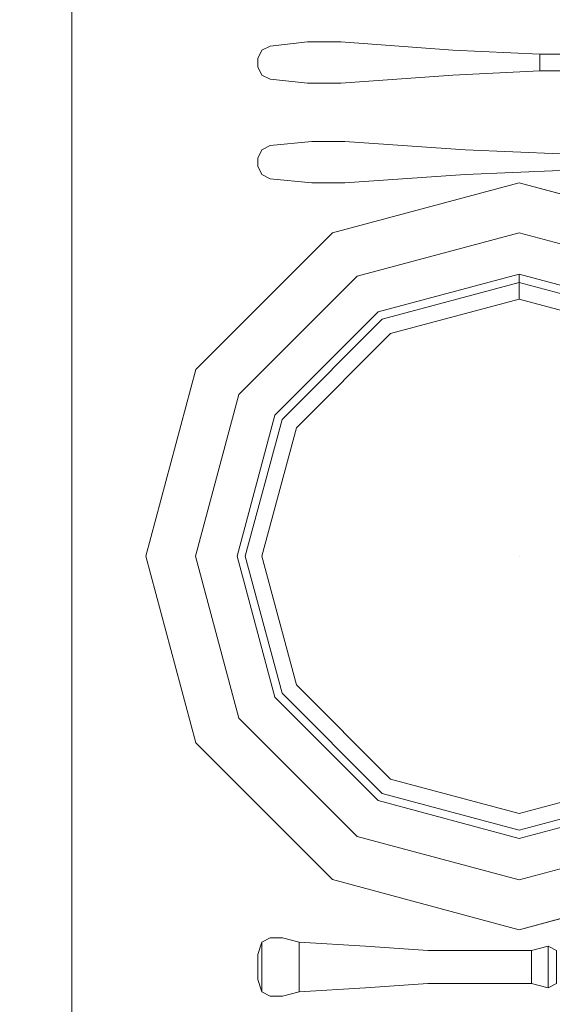
# Model space of a CAD drawing. Units: inches. Extents: x 375 to 1122, y 27 to 1069.
# Tile 18 of 155: x 705.14 to 713.05, y 270.59 to 285.2. Entities that reach past the tile are written whole.
import ezdxf

# ---------------------------------------------------------------- set-up
doc = ezdxf.new("R2010")
doc.units = ezdxf.units.IN
doc.layers.add('A-ANNO-DIMS', color=2, linetype='Continuous', lineweight=18)
doc.layers.add('Furniture', color=30, linetype='Continuous', lineweight=18)
doc.styles.get("Standard").update_dxf_attribs({"font": 'arial.ttf'})
doc.dimstyles.new('ISO-25', dxfattribs={"dimtxt": 12, "dimasz": 2.5, "dimexe": 1.5, "dimexo": 1.5, "dimtad": 1, "dimdec": 1, "dimlunit": 3, "dimtxsty": 'Standard', "dimblk": 'ARCHTICK', "dimcen": 2.5, "dimadec": 0, "dimazin": 0, "dimtfac": 1, "dimtdec": 1, "dimtmove": 0, "dimatfit": 3, "dimfxl": 1.5, "dimfxlon": 1, "dimarcsym": 0})

# ---------------------------------------------------------------- blocks, each defined once
blk = doc.blocks.new('A$C403C54AD')
blk.add_line((0.83575, 0.52421, -0.0006), (1.99923, 0.52421, -0.0006))
at = {"linetype": 'ByBlock'}
for points, invisible_edges in [([(1.72651, 0.7917, -0.01489), (1.72651, 0.69011, -0.01489), (1.72651, 0.69011, -0.01489), (1.67572, 0.77809, -0.01489)], 5), ([(1.7773, 0.77809, -0.01489), (1.72651, 0.69011, -0.01489), (1.72651, 0.69011, -0.01489), (1.72651, 0.7917, -0.01489)], 5), ([(1.67572, 0.77809, -0.01489), (1.72651, 0.69011, -0.01489), (1.72651, 0.69011, -0.01489), (1.63853, 0.74091, -0.01489)], 5), ([(1.81449, 0.74091, -0.01489), (1.72651, 0.69011, -0.01489), (1.72651, 0.69011, -0.01489), (1.7773, 0.77809, -0.01489)], 5), ([(1.60654, 0.75938, -0.00874), (1.62254, 0.75014, -0.00874), (1.60645, 0.69011, -0.00874), (1.58798, 0.69011, -0.00874)], 5), ([(1.63587, 0.74244, -0.02259), (1.60654, 0.75938, -0.01335), (1.58798, 0.69011, -0.01335), (1.62185, 0.69011, -0.02259)], 5), ([(1.83118, 0.69011, -0.02259), (1.86504, 0.69011, -0.01335), (1.84648, 0.75938, -0.01335), (1.81715, 0.74244, -0.02259)], 5), ([(1.86504, 0.69011, -0.00874), (1.84657, 0.69011, -0.00874), (1.83048, 0.75014, -0.00874), (1.84648, 0.75938, -0.00874)], 5), ([(1.62254, 0.75014, -0.00874), (1.63853, 0.74091, -0.01489), (1.62492, 0.69011, -0.01489), (1.60645, 0.69011, -0.00874)], 5), ([(1.84657, 0.69011, -0.00874), (1.8281, 0.69011, -0.01489), (1.81449, 0.74091, -0.01489), (1.83048, 0.75014, -0.00874)], 5), ([(1.82194, 0.69011, -0.03183), (1.83118, 0.69011, -0.02259), (1.81715, 0.74244, -0.02259), (1.80916, 0.73783, -0.03183)], 5), ([(1.63853, 0.74091, -0.01489), (1.72651, 0.69011, -0.01489), (1.72651, 0.69011, -0.01489), (1.62492, 0.69011, -0.01489)], 5), ([(1.8281, 0.69011, -0.01489), (1.72651, 0.69011, -0.01489), (1.72651, 0.69011, -0.01489), (1.81449, 0.74091, -0.01489)], 5), ([(1.58798, 0.69011, -0.00874), (1.60645, 0.69011, -0.00874), (1.62254, 0.63008, -0.00874), (1.60654, 0.62085, -0.00874)], 5), ([(1.62185, 0.69011, -0.02259), (1.58798, 0.69011, -0.01335), (1.60654, 0.62085, -0.01335), (1.63587, 0.63778, -0.02259)], 5), ([(1.60645, 0.69011, -0.00874), (1.62492, 0.69011, -0.01489), (1.63853, 0.63932, -0.01489), (1.62254, 0.63008, -0.00874)], 5), ([(1.63108, 0.69011, -0.03183), (1.62185, 0.69011, -0.02259), (1.63587, 0.63778, -0.02259), (1.64387, 0.6424, -0.03183)], 4), ([(1.62492, 0.69011, -0.01489), (1.72651, 0.69011, -0.01489), (1.72651, 0.69011, -0.01489), (1.63853, 0.63932, -0.01489)], 5), ([(1.63853, 0.63932, -0.01489), (1.72651, 0.69011, -0.01489), (1.72651, 0.69011, -0.01489), (1.67572, 0.60214, -0.01489)], 5), ([(1.67572, 0.60214, -0.01489), (1.72651, 0.69011, -0.01489), (1.72651, 0.69011, -0.01489), (1.72651, 0.58853, -0.01489)], 5), ([(1.72651, 0.58853, -0.01489), (1.72651, 0.69011, -0.01489), (1.72651, 0.69011, -0.01489), (1.7773, 0.60214, -0.01489)], 5), ([(1.7773, 0.60214, -0.01489), (1.72651, 0.69011, -0.01489), (1.72651, 0.69011, -0.01489), (1.81449, 0.63932, -0.01489)], 5), ([(1.81449, 0.63932, -0.01489), (1.72651, 0.69011, -0.01489), (1.72651, 0.69011, -0.01489), (1.8281, 0.69011, -0.01489)], 5), ([(1.80916, 0.6424, -0.03183), (1.81715, 0.63778, -0.02259), (1.83118, 0.69011, -0.02259), (1.82194, 0.69011, -0.03183)], 5), ([(1.83048, 0.63008, -0.00874), (1.81449, 0.63932, -0.01489), (1.8281, 0.69011, -0.01489), (1.84657, 0.69011, -0.00874)], 5), ([(1.81715, 0.63778, -0.02259), (1.84648, 0.62085, -0.01335), (1.86504, 0.69011, -0.01335), (1.83118, 0.69011, -0.02259)], 5), ([(1.84648, 0.62085, -0.00874), (1.83048, 0.63008, -0.00874), (1.84657, 0.69011, -0.00874), (1.86504, 0.69011, -0.00874)], 5), ([(1.62254, 0.63008, -0.00874), (1.63853, 0.63932, -0.01489), (1.67572, 0.60214, -0.01489), (1.66648, 0.58614, -0.00874)], 5), ([(1.64387, 0.6424, -0.03183), (1.63587, 0.63778, -0.02259), (1.67418, 0.59947, -0.02259), (1.6788, 0.60747, -0.03183)], 5), ([(1.77423, 0.60747, -0.03183), (1.77884, 0.59947, -0.02259), (1.81715, 0.63778, -0.02259), (1.80916, 0.6424, -0.03183)], 5), ([(1.78654, 0.58614, -0.00874), (1.7773, 0.60214, -0.01489), (1.81449, 0.63932, -0.01489), (1.83048, 0.63008, -0.00874)], 5), ([(1.63587, 0.63778, -0.02259), (1.60654, 0.62085, -0.01335), (1.65725, 0.57014, -0.01335), (1.67418, 0.59947, -0.02259)], 5), ([(1.77884, 0.59947, -0.02259), (1.79578, 0.57014, -0.01335), (1.84648, 0.62085, -0.01335), (1.81715, 0.63778, -0.02259)], 5), ([(1.60654, 0.62085, -0.00874), (1.62254, 0.63008, -0.00874), (1.66648, 0.58614, -0.00874), (1.65725, 0.57014, -0.00874)], 5), ([(1.79578, 0.57014, -0.00874), (1.78654, 0.58614, -0.00874), (1.83048, 0.63008, -0.00874), (1.84648, 0.62085, -0.00874)], 5), ([(1.6788, 0.60747, -0.03183), (1.67418, 0.59947, -0.02259), (1.72651, 0.58545, -0.02259), (1.72651, 0.59468, -0.03183)], 5), ([(1.72651, 0.59468, -0.03183), (1.72651, 0.58545, -0.02259), (1.77884, 0.59947, -0.02259), (1.77423, 0.60747, -0.03183)], 5), ([(1.67418, 0.59947, -0.02259), (1.65725, 0.57014, -0.01335), (1.72651, 0.55159, -0.01335), (1.72651, 0.58545, -0.02259)], 5), ([(1.66648, 0.58614, -0.00874), (1.67572, 0.60214, -0.01489), (1.72651, 0.58853, -0.01489), (1.72651, 0.57006, -0.00874)], 5), ([(1.72651, 0.57006, -0.00874), (1.72651, 0.58853, -0.01489), (1.7773, 0.60214, -0.01489), (1.78654, 0.58614, -0.00874)], 5), ([(1.72651, 0.58545, -0.02259), (1.72651, 0.55159, -0.01335), (1.79578, 0.57014, -0.01335), (1.77884, 0.59947, -0.02259)], 5), ([(1.65725, 0.57014, -0.00874), (1.66648, 0.58614, -0.00874), (1.72651, 0.57006, -0.00874), (1.72651, 0.55159, -0.00874)], 5), ([(1.72651, 0.55159, -0.00874), (1.72651, 0.57006, -0.00874), (1.78654, 0.58614, -0.00874), (1.79578, 0.57014, -0.00874)], 5)]:
    blk.add_3dface(points, dxfattribs=dict(at, invisible_edges=invisible_edges))
for points in [[(1.60654, 0.75938, -0.01335), (1.60654, 0.75938, -0.00874), (1.58798, 0.69011, -0.00874), (1.58798, 0.69011, -0.01335)], [(1.86504, 0.69011, -0.01335), (1.86504, 0.69011, -0.00874), (1.84648, 0.75938, -0.00874), (1.84648, 0.75938, -0.01335)], [(1.64387, 0.73783, -0.03183), (1.63587, 0.74244, -0.02259), (1.62185, 0.69011, -0.02259), (1.63108, 0.69011, -0.03183)], [(1.58798, 0.69011, -0.01335), (1.58798, 0.69011, -0.00874), (1.60654, 0.62085, -0.00874), (1.60654, 0.62085, -0.01335)], [(1.84648, 0.62085, -0.01335), (1.84648, 0.62085, -0.00874), (1.86504, 0.69011, -0.00874), (1.86504, 0.69011, -0.01335)], [(1.60654, 0.62085, -0.01335), (1.60654, 0.62085, -0.00874), (1.65725, 0.57014, -0.00874), (1.65725, 0.57014, -0.01335)], [(1.79578, 0.57014, -0.01335), (1.79578, 0.57014, -0.00874), (1.84648, 0.62085, -0.00874), (1.84648, 0.62085, -0.01335)], [(1.65725, 0.57014, -0.01335), (1.65725, 0.57014, -0.00874), (1.72651, 0.55159, -0.00874), (1.72651, 0.55159, -0.01335)], [(1.72651, 0.55159, -0.01335), (1.72651, 0.55159, -0.00874), (1.79578, 0.57014, -0.00874), (1.79578, 0.57014, -0.01335)]]:
    blk.add_3dface(points, dxfattribs=at)
for points in [[(1.54027, 0.69781, -0.01387), (1.54643, 0.69781, -0.01387), (1.54643, 0.70858, -0.01595), (1.54027, 0.70858, -0.01595)], [(1.54027, 0.69781, -0.01646), (1.54643, 0.69781, -0.01646), (1.54643, 0.70858, -0.01854), (1.54027, 0.70858, -0.01854)], [(1.87273, 0.70396, -0.02105), (1.88505, 0.70396, -0.02105), (1.88659, 0.70089, -0.01951), (1.8712, 0.70089, -0.01951)], [(1.87273, 0.70396, -0.03029), (1.88505, 0.70396, -0.03029), (1.88659, 0.70089, -0.03183), (1.8712, 0.70089, -0.03183)], [(1.87273, 0.70396, -0.02105), (1.87273, 0.70396, -0.03029), (1.8712, 0.70089, -0.03183), (1.8712, 0.70089, -0.01951)], [(1.88659, 0.70089, -0.01951), (1.88659, 0.70089, -0.03183), (1.88505, 0.70396, -0.03029), (1.88505, 0.70396, -0.02105)], [(1.88659, 0.70089, -0.01951), (1.8712, 0.70089, -0.01951), (1.87273, 0.69473, -0.02105), (1.88505, 0.69473, -0.02105)], [(1.88659, 0.70089, -0.03183), (1.8712, 0.70089, -0.03183), (1.87273, 0.69473, -0.03029), (1.88505, 0.69473, -0.03029)], [(1.8712, 0.70089, -0.03183), (1.8712, 0.70089, -0.01951), (1.87273, 0.69473, -0.02105), (1.87273, 0.69473, -0.03029)], [(1.88505, 0.69473, -0.03029), (1.88505, 0.69473, -0.02105), (1.88659, 0.70089, -0.01951), (1.88659, 0.70089, -0.03183)], [(1.87273, 0.69473, -0.02105), (1.87273, 0.69473, -0.03029), (1.87273, 0.65625, -0.03183), (1.87273, 0.65625, -0.01951)], [(1.88505, 0.65625, -0.01951), (1.88505, 0.65625, -0.03183), (1.88505, 0.69473, -0.03029), (1.88505, 0.69473, -0.02105)], [(1.87273, 0.65625, -0.03183), (1.87273, 0.65625, -0.01951), (1.8712, 0.63316, -0.01951), (1.8712, 0.63316, -0.03183)], [(1.88659, 0.63316, -0.03183), (1.88659, 0.63316, -0.01951), (1.88505, 0.65625, -0.01951), (1.88505, 0.65625, -0.03183)], [(1.8712, 0.63316, -0.01951), (1.8712, 0.63316, -0.03183), (1.86966, 0.60854, -0.03029), (1.86966, 0.60854, -0.02105)], [(1.88813, 0.60854, -0.02105), (1.88813, 0.60854, -0.03029), (1.88659, 0.63316, -0.03183), (1.88659, 0.63316, -0.01951)], [(1.57259, 0.62547, -0.01916), (1.57259, 0.62547, -0.0238), (1.57259, 0.61315, -0.02413), (1.57259, 0.61315, -0.01949)], [(1.58798, 0.61315, -0.01949), (1.58798, 0.61315, -0.02413), (1.58798, 0.62547, -0.0238), (1.58798, 0.62547, -0.01916)], [(1.53565, 0.62393, -0.01916), (1.53565, 0.62393, -0.0238), (1.53565, 0.61161, -0.02413), (1.53565, 0.61161, -0.01949)], [(1.55104, 0.61161, -0.01949), (1.55104, 0.61161, -0.02413), (1.55104, 0.62393, -0.0238), (1.55104, 0.62393, -0.01916)], [(1.53565, 0.61161, -0.02413), (1.53565, 0.61161, -0.01949), (1.53719, 0.59776, -0.01946), (1.53719, 0.59776, -0.02409)], [(1.5495, 0.59776, -0.02409), (1.5495, 0.59776, -0.01946), (1.55104, 0.61161, -0.01949), (1.55104, 0.61161, -0.02413)], [(1.57259, 0.61315, -0.02413), (1.57259, 0.61315, -0.01949), (1.57413, 0.59776, -0.01946), (1.57413, 0.59776, -0.02409)], [(1.58645, 0.59776, -0.02409), (1.58645, 0.59776, -0.01946), (1.58798, 0.61315, -0.01949), (1.58798, 0.61315, -0.02413)], [(1.86966, 0.60854, -0.03029), (1.86966, 0.60854, -0.02105), (1.86812, 0.60238, -0.01951), (1.86812, 0.60238, -0.03183)], [(1.88967, 0.60238, -0.03183), (1.88967, 0.60238, -0.01951), (1.88813, 0.60854, -0.02105), (1.88813, 0.60854, -0.03029)], [(1.86812, 0.60238, -0.01951), (1.86812, 0.60238, -0.03183), (1.86812, 0.59776, -0.03029), (1.86812, 0.59776, -0.02105)], [(1.88967, 0.59776, -0.02105), (1.88967, 0.59776, -0.03029), (1.88967, 0.60238, -0.03183), (1.88967, 0.60238, -0.01951)], [(1.53719, 0.59776, -0.01946), (1.53719, 0.59776, -0.02409), (1.53873, 0.59468, -0.02385), (1.53873, 0.59468, -0.01921)], [(1.54797, 0.59468, -0.01921), (1.54797, 0.59468, -0.02385), (1.5495, 0.59776, -0.02409), (1.5495, 0.59776, -0.01946)], [(1.57413, 0.59776, -0.01946), (1.57413, 0.59776, -0.02409), (1.57567, 0.59468, -0.02385), (1.57567, 0.59468, -0.01921)], [(1.58491, 0.59468, -0.01921), (1.58491, 0.59468, -0.02385), (1.58645, 0.59776, -0.02409), (1.58645, 0.59776, -0.01946)], [(1.86812, 0.59776, -0.03029), (1.86812, 0.59776, -0.02105), (1.86966, 0.59468, -0.02259), (1.86966, 0.59468, -0.02875)], [(1.88813, 0.59468, -0.02259), (1.88813, 0.59468, -0.02875), (1.88967, 0.59776, -0.03029), (1.88967, 0.59776, -0.02105)], [(1.53873, 0.59468, -0.02385), (1.53873, 0.59468, -0.01921), (1.54181, 0.59314, -0.01938), (1.54181, 0.59314, -0.02351)], [(1.54181, 0.59314, -0.01938), (1.54181, 0.59314, -0.02351), (1.54489, 0.59314, -0.02351), (1.54489, 0.59314, -0.01938)], [(1.54489, 0.59314, -0.02351), (1.54489, 0.59314, -0.01938), (1.54797, 0.59468, -0.01921), (1.54797, 0.59468, -0.02385)], [(1.57567, 0.59468, -0.02385), (1.57567, 0.59468, -0.01921), (1.57875, 0.59314, -0.01938), (1.57875, 0.59314, -0.02351)], [(1.57875, 0.59314, -0.01938), (1.57875, 0.59314, -0.02351), (1.58183, 0.59314, -0.02351), (1.58183, 0.59314, -0.01938)], [(1.58183, 0.59314, -0.02351), (1.58183, 0.59314, -0.01938), (1.58491, 0.59468, -0.01921), (1.58491, 0.59468, -0.02385)], [(1.86966, 0.59468, -0.02259), (1.88813, 0.59468, -0.02259), (1.88351, 0.59314, -0.02567), (1.87427, 0.59314, -0.02567)], [(1.86966, 0.59468, -0.02259), (1.86966, 0.59468, -0.02875), (1.87427, 0.59314, -0.02567)], [(1.86966, 0.59468, -0.02875), (1.88813, 0.59468, -0.02875), (1.88351, 0.59314, -0.02567), (1.87427, 0.59314, -0.02567)], [(1.88351, 0.59314, -0.02567), (1.88351, 0.59314, -0.02567), (1.88813, 0.59468, -0.02259), (1.88813, 0.59468, -0.02875)]]:
    blk.add_3dface(points)
for points, invisible_edges in [([(1.54027, 0.70858, -0.01854), (1.54027, 0.70858, -0.01595), (1.54027, 0.69781, -0.01387), (1.54027, 0.69781, -0.01646)], 5), ([(1.54643, 0.69781, -0.01646), (1.54643, 0.69781, -0.01387), (1.54643, 0.70858, -0.01595), (1.54643, 0.70858, -0.01854)], 5), ([(1.58491, 0.6701, -0.01678), (1.57567, 0.6701, -0.01678), (1.57721, 0.7055, -0.01387), (1.58337, 0.7055, -0.01387)], 1), ([(1.57721, 0.7055, -0.01387), (1.57721, 0.7055, -0.01646), (1.57567, 0.6701, -0.01986), (1.57567, 0.6701, -0.01678)], 5), ([(1.58491, 0.6701, -0.01986), (1.57567, 0.6701, -0.01986), (1.57721, 0.7055, -0.01646), (1.58337, 0.7055, -0.01646)], 1), ([(1.58491, 0.6701, -0.01678), (1.58491, 0.6701, -0.01986), (1.58337, 0.7055, -0.01646), (1.58337, 0.7055, -0.01387)], 5), ([(1.54797, 0.66549, -0.01678), (1.53873, 0.66549, -0.01678), (1.54027, 0.69781, -0.01387), (1.54643, 0.69781, -0.01387)], 1), ([(1.54027, 0.69781, -0.01387), (1.54027, 0.69781, -0.01646), (1.53873, 0.66549, -0.01986), (1.53873, 0.66549, -0.01678)], 5), ([(1.54797, 0.66549, -0.01986), (1.53873, 0.66549, -0.01986), (1.54027, 0.69781, -0.01646), (1.54643, 0.69781, -0.01646)], 1), ([(1.54797, 0.66549, -0.01678), (1.54797, 0.66549, -0.01986), (1.54643, 0.69781, -0.01646), (1.54643, 0.69781, -0.01387)], 5), ([(1.87273, 0.69473, -0.02105), (1.88505, 0.69473, -0.02105), (1.88505, 0.65625, -0.01951), (1.87273, 0.65625, -0.01951)], 4), ([(1.87273, 0.69473, -0.03029), (1.88505, 0.69473, -0.03029), (1.88505, 0.65625, -0.03183), (1.87273, 0.65625, -0.03183)], 4), ([(1.57259, 0.62547, -0.01916), (1.58798, 0.62547, -0.01916), (1.58491, 0.6701, -0.01678), (1.57567, 0.6701, -0.01678)], 5), ([(1.57259, 0.62547, -0.0238), (1.58798, 0.62547, -0.0238), (1.58491, 0.6701, -0.01986), (1.57567, 0.6701, -0.01986)], 5), ([(1.57567, 0.6701, -0.01986), (1.57567, 0.6701, -0.01678), (1.57259, 0.62547, -0.01916), (1.57259, 0.62547, -0.0238)], 1), ([(1.58798, 0.62547, -0.0238), (1.58798, 0.62547, -0.01916), (1.58491, 0.6701, -0.01678), (1.58491, 0.6701, -0.01986)], 4), ([(1.53565, 0.62393, -0.01916), (1.55104, 0.62393, -0.01916), (1.54797, 0.66549, -0.01678), (1.53873, 0.66549, -0.01678)], 5), ([(1.53565, 0.62393, -0.0238), (1.55104, 0.62393, -0.0238), (1.54797, 0.66549, -0.01986), (1.53873, 0.66549, -0.01986)], 5), ([(1.53873, 0.66549, -0.01986), (1.53873, 0.66549, -0.01678), (1.53565, 0.62393, -0.01916), (1.53565, 0.62393, -0.0238)], 1), ([(1.55104, 0.62393, -0.0238), (1.55104, 0.62393, -0.01916), (1.54797, 0.66549, -0.01678), (1.54797, 0.66549, -0.01986)], 4), ([(1.88505, 0.65625, -0.01951), (1.87273, 0.65625, -0.01951), (1.8712, 0.63316, -0.01951), (1.88659, 0.63316, -0.01951)], 5), ([(1.88505, 0.65625, -0.03183), (1.87273, 0.65625, -0.03183), (1.8712, 0.63316, -0.03183), (1.88659, 0.63316, -0.03183)], 5), ([(1.8712, 0.63316, -0.01951), (1.88659, 0.63316, -0.01951), (1.88813, 0.60854, -0.02105), (1.86966, 0.60854, -0.02105)], 1), ([(1.8712, 0.63316, -0.03183), (1.88659, 0.63316, -0.03183), (1.88813, 0.60854, -0.03029), (1.86966, 0.60854, -0.03029)], 1), ([(1.58798, 0.61315, -0.01949), (1.57259, 0.61315, -0.01949), (1.57259, 0.62547, -0.01916), (1.58798, 0.62547, -0.01916)], 5), ([(1.58798, 0.61315, -0.02413), (1.57259, 0.61315, -0.02413), (1.57259, 0.62547, -0.0238), (1.58798, 0.62547, -0.0238)], 5), ([(1.55104, 0.61161, -0.01949), (1.53565, 0.61161, -0.01949), (1.53565, 0.62393, -0.01916), (1.55104, 0.62393, -0.01916)], 5), ([(1.55104, 0.61161, -0.02413), (1.53565, 0.61161, -0.02413), (1.53565, 0.62393, -0.0238), (1.55104, 0.62393, -0.0238)], 5), ([(1.53719, 0.59776, -0.01946), (1.5495, 0.59776, -0.01946), (1.55104, 0.61161, -0.01949), (1.53565, 0.61161, -0.01949)], 5), ([(1.53719, 0.59776, -0.02409), (1.5495, 0.59776, -0.02409), (1.55104, 0.61161, -0.02413), (1.53565, 0.61161, -0.02413)], 5), ([(1.57413, 0.59776, -0.01946), (1.58645, 0.59776, -0.01946), (1.58798, 0.61315, -0.01949), (1.57259, 0.61315, -0.01949)], 5), ([(1.57413, 0.59776, -0.02409), (1.58645, 0.59776, -0.02409), (1.58798, 0.61315, -0.02413), (1.57259, 0.61315, -0.02413)], 5), ([(1.88813, 0.60854, -0.02105), (1.86966, 0.60854, -0.02105), (1.86812, 0.60238, -0.01951), (1.88967, 0.60238, -0.01951)], 4), ([(1.88813, 0.60854, -0.03029), (1.86966, 0.60854, -0.03029), (1.86812, 0.60238, -0.03183), (1.88967, 0.60238, -0.03183)], 4), ([(1.86812, 0.60238, -0.01951), (1.88967, 0.60238, -0.01951), (1.88967, 0.59776, -0.02105), (1.86812, 0.59776, -0.02105)], 5), ([(1.86812, 0.60238, -0.03183), (1.88967, 0.60238, -0.03183), (1.88967, 0.59776, -0.03029), (1.86812, 0.59776, -0.03029)], 5), ([(1.54797, 0.59468, -0.01921), (1.53873, 0.59468, -0.01921), (1.53719, 0.59776, -0.01946), (1.5495, 0.59776, -0.01946)], 5), ([(1.54797, 0.59468, -0.02385), (1.53873, 0.59468, -0.02385), (1.53719, 0.59776, -0.02409), (1.5495, 0.59776, -0.02409)], 5), ([(1.58491, 0.59468, -0.01921), (1.57567, 0.59468, -0.01921), (1.57413, 0.59776, -0.01946), (1.58645, 0.59776, -0.01946)], 5), ([(1.58491, 0.59468, -0.02385), (1.57567, 0.59468, -0.02385), (1.57413, 0.59776, -0.02409), (1.58645, 0.59776, -0.02409)], 5), ([(1.88967, 0.59776, -0.02105), (1.86812, 0.59776, -0.02105), (1.86966, 0.59468, -0.02259), (1.88813, 0.59468, -0.02259)], 1), ([(1.88967, 0.59776, -0.03029), (1.86812, 0.59776, -0.03029), (1.86966, 0.59468, -0.02875), (1.88813, 0.59468, -0.02875)], 1), ([(1.54181, 0.59314, -0.01938), (1.54489, 0.59314, -0.01938), (1.54797, 0.59468, -0.01921), (1.53873, 0.59468, -0.01921)], 4), ([(1.54181, 0.59314, -0.02351), (1.54489, 0.59314, -0.02351), (1.54797, 0.59468, -0.02385), (1.53873, 0.59468, -0.02385)], 4), ([(1.57875, 0.59314, -0.01938), (1.58183, 0.59314, -0.01938), (1.58491, 0.59468, -0.01921), (1.57567, 0.59468, -0.01921)], 4), ([(1.57875, 0.59314, -0.02351), (1.58183, 0.59314, -0.02351), (1.58491, 0.59468, -0.02385), (1.57567, 0.59468, -0.02385)], 4)]:
    blk.add_3dface(points, dxfattribs=dict(invisible_edges=invisible_edges))
blk = doc.blocks.new('_ArchTick')
at = {"color": 0, "linetype": 'ByBlock', "const_width": 0.15}
blk.add_lwpolyline([(-0.5, -0.5), (0.5, 0.5)], dxfattribs=at)
blk = doc.blocks.new('*D59')
at = {"layer": 'A-ANNO-DIMS', "color": 0, "lineweight": -2, "transparency": 16777216}
for p, q in [((668.717, 346.851), (665.717, 346.851)), ((667.217, 346.851), (667.217, 232.348)), ((668.717, 232.348), (665.717, 232.348)), ((667.217, 232.348), (667.217, 27.496))]:
    blk.add_line(p, q, dxfattribs=at)
at = {"layer": 'Defpoints', "color": 0, "transparency": 16777216}
for p in [(684.392, 346.851), (667.217, 232.348), (684.392, 232.348)]:
    blk.add_point(p, dxfattribs=at)
at = {"layer": 'A-ANNO-DIMS', "color": 0, "lineweight": -2, "transparency": 16777216, "xscale": 2.5, "yscale": 2.5, "zscale": 2.5}
for p, rotation in [((667.217, 346.851), 90), ((667.217, 232.348), 270)]:
    blk.add_blockref('_ArchTick', p, dxfattribs=dict(at, rotation=rotation))
at = {"layer": 'A-ANNO-DIMS', "color": 0, "transparency": 16777216, "insert": (660.387, 128.672), "char_height": 12, "attachment_point": 5, "rotation": 90}
blk.add_mtext('DINING SET 9\'-6 1/2" TYP.', dxfattribs=at)

msp = doc.modelspace()

# ---------------------------------------------------------------- block references
at = {"layer": 'Furniture', "xscale": 39.9918517141215, "yscale": 39.9918517141215, "zscale": 39.9918517141215, "rotation": 270}
msp.add_blockref('A$C403C54AD', (684.955, 346.287, 0.024), dxfattribs=at)

# ---------------------------------------------------------------- dimensions: what is measured, and where the dimension line sits
at = {"layer": 'A-ANNO-DIMS'}
dim = msp.add_linear_dim(base=(667.217, 232.348), p1=(684.392, 346.851), p2=(684.392, 232.348), angle=270, text='DINING SET <> TYP.', dimstyle='ISO-25', override={"dimdec": 1, "dimlfac": 1, "dimrnd": 0, "dimzin": 1, "dimdsep": 46, "dimlunit": 4, "dimfrac": 2}, dxfattribs=at)
dim.commit()
dim.dimension.update_dxf_attribs({"geometry": '*D59', "text_midpoint": (660.387, 128.672)})

doc.saveas('drawing.dxf')
